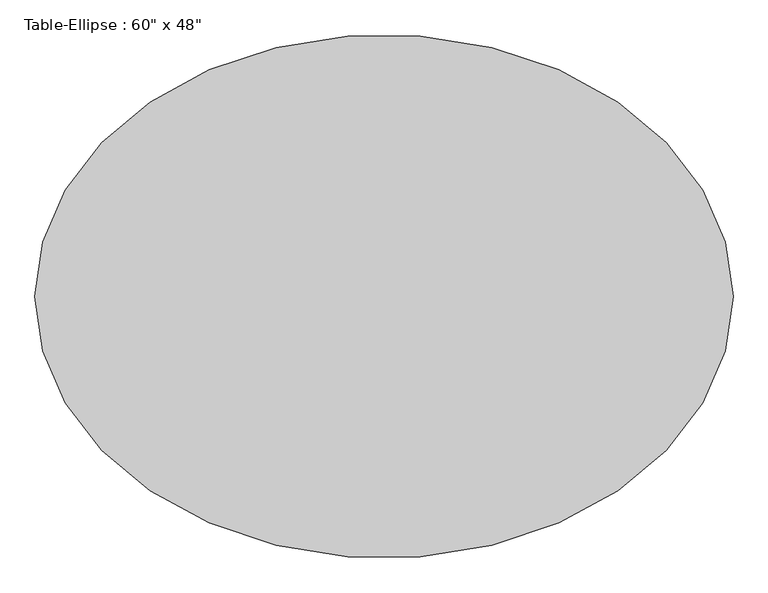
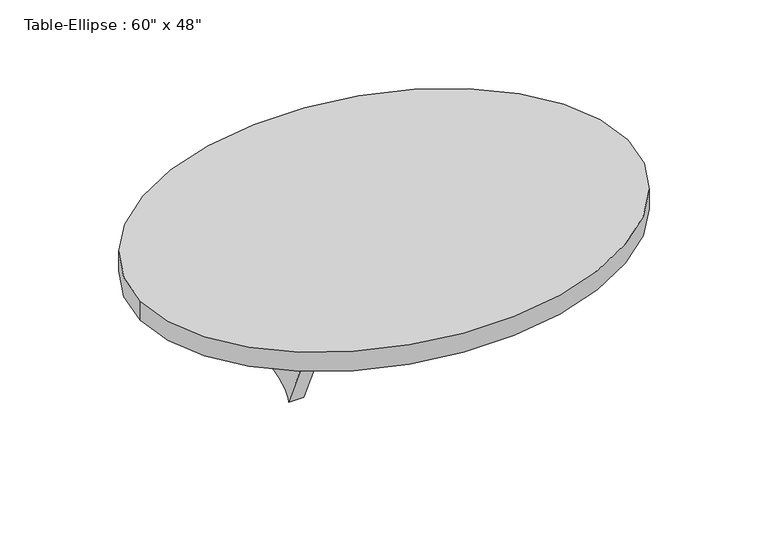
"""IFC4 building model written with IfcOpenShell, lengths in millimetres: furniture geometry."""

from ifc_helpers import new_model, si_unit, point, frame, origin, place, context, project, spatial, ellipse_curve, trimmed, source, transform, mapped, element, save
from ifc_brep_helpers import plane_surface, extruded_surface, advanced_brep


def furniture_b94c68a7(model_context):
    return source(origin(), model_context, "Body", "AdvancedBrep", [
        advanced_brep(
        [(-609.6, 0.0, 304.8), (609.6, 0.0, 304.8), (-609.6, 0.0, 254.0), (609.6, 0.0, 254.0)],
        [
            (0, 1, ellipse_curve(frame((0.0, 0.0, 304.8), z_axis=(0.0, 0.0, 1.0), x_axis=(1.0, 0.0, 0.0)), 609.6, 457.2)),
            (1, 0, ellipse_curve(frame((0.0, 0.0, 304.8), z_axis=(0.0, 0.0, 1.0), x_axis=(1.0, 0.0, 0.0)), 609.6, 457.2)),
            (2, 3, ellipse_curve(frame((0.0, 0.0, 254.0), z_axis=(0.0, 0.0, -1.0), x_axis=(1.0, 0.0, 0.0)), 609.6, 457.2)),
            (3, 2, ellipse_curve(frame((0.0, 0.0, 254.0), z_axis=(0.0, 0.0, -1.0), x_axis=(1.0, 0.0, 0.0)), 609.6, 457.2)),
            (0, 2),
            (3, 1),
        ],
        [
            plane_surface(frame((609.6, 0.0, 304.8), z_axis=(0.0, 0.0, 1.0), x_axis=(0.0, 1.0, 0.0))),
            plane_surface(frame((609.6, 0.0, 254.0), z_axis=(0.0, 0.0, -1.0), x_axis=(0.0, -1.0, 0.0))),
            extruded_surface(trimmed(ellipse_curve(frame((0.0, 0.0, 203.2), z_axis=(0.0, 0.0, 1.0), x_axis=(1.0, 0.0, 0.0)), 609.6, 457.2), [point((-609.6, 0.0, 203.2))], [point((609.6, 0.0, 203.2))], True, "CARTESIAN"), (0.0, 0.0, 50.80000000000001), 50.80000000000001),
            extruded_surface(trimmed(ellipse_curve(frame((0.0, 0.0, 203.2), z_axis=(0.0, 0.0, 1.0), x_axis=(1.0, 0.0, 0.0)), 609.6, 457.2), [point((609.6, 0.0, 203.2))], [point((-609.6, 0.0, 203.2))], True, "CARTESIAN"), (0.0, 0.0, 50.80000000000001), 50.80000000000001),
        ],
        [
            (0, [[1, 2]]),
            (1, [[3, 4]]),
            (2, [[-1, 5, -4, 6]]),
            (3, [[-2, -6, -3, -5]]),
        ],
    ),
        advanced_brep(
        [(-266.7, 228.6, 254.0), (-266.7, -228.6, 254.0), (-266.7, -114.3, 0.0), (-266.7, 114.3, 0.0), (-304.8, 228.6, 254.0), (-304.8, 114.3, 0.0), (-304.8, -114.3, 0.0), (-304.8, -228.6, 254.0)],
        [
            (0, 1),
            (1, 2),
            (2, 3, ellipse_curve(frame((-266.7, 0.0, 0.0), z_axis=(-1.0, 0.0, 0.0), x_axis=(0.0, 1.0, 0.0)), 114.3, 50.8)),
            (3, 0),
            (4, 5),
            (5, 6, ellipse_curve(frame((-304.8, 0.0, 0.0), z_axis=(1.0, 0.0, 0.0), x_axis=(0.0, 1.0, 0.0)), 114.3, 50.8)),
            (6, 7),
            (7, 4),
            (0, 4),
            (7, 1),
            (6, 2),
            (5, 3),
        ],
        [
            plane_surface(frame((-266.7, -228.6, 254.0), z_axis=(1.0, 0.0, 0.0), x_axis=(0.0, -1.0, 0.0))),
            plane_surface(frame((-304.8, -228.6, 254.0), z_axis=(-1.0, 0.0, 0.0), x_axis=(0.0, 1.0, 0.0))),
            plane_surface(frame((-266.7, 228.6, 254.0), z_axis=(0.0, 0.0, 1.0), x_axis=(-1.0, 0.0, 0.0))),
            plane_surface(frame((-266.7, -228.6, 254.0), z_axis=(0.0, -0.9119215051750983, -0.410364677328816), x_axis=(-1.0, 0.0, 0.0))),
            extruded_surface(trimmed(ellipse_curve(frame((-342.9, 0.0, 0.0), z_axis=(-1.0, 0.0, 0.0), x_axis=(0.0, 1.0, 0.0)), 114.3, 50.8), [point((-342.9, -114.3, 0.0))], [point((-342.9, 114.3, 0.0))], True, "CARTESIAN"), (38.099999999999966, 0.0, 0.0), 38.099999999999966),
            plane_surface(frame((-266.7, 114.3, 0.0), z_axis=(0.0, 0.911921505175108, -0.41036467732879445), x_axis=(-1.0, 0.0, 0.0))),
        ],
        [
            (0, [[1, 2, 3, 4]]),
            (1, [[5, 6, 7, 8]]),
            (2, [[-1, 9, -8, 10]]),
            (3, [[-2, -10, -7, 11]]),
            (4, [[-3, -11, -6, 12]]),
            (5, [[-4, -12, -5, -9]]),
        ],
    ),
        advanced_brep(
        [(304.8, 228.6, 254.0), (304.8, -228.6, 254.0), (304.8, -114.3, 0.0), (304.8, 114.3, 0.0), (266.7, 228.6, 254.0), (266.7, 114.3, 0.0), (266.7, -114.3, 0.0), (266.7, -228.6, 254.0)],
        [
            (0, 1),
            (1, 2),
            (2, 3, ellipse_curve(frame((304.8, 0.0, 0.0), z_axis=(-1.0, 0.0, 0.0), x_axis=(0.0, 1.0, 0.0)), 114.3, 50.8)),
            (3, 0),
            (4, 5),
            (5, 6, ellipse_curve(frame((266.7, 0.0, 0.0), z_axis=(1.0, 0.0, 0.0), x_axis=(0.0, 1.0, 0.0)), 114.3, 50.8)),
            (6, 7),
            (7, 4),
            (0, 4),
            (7, 1),
            (6, 2),
            (5, 3),
        ],
        [
            plane_surface(frame((304.8, -228.6, 254.0), z_axis=(1.0, 0.0, 0.0), x_axis=(0.0, -1.0, 0.0))),
            plane_surface(frame((266.7, -228.6, 254.0), z_axis=(-1.0, 0.0, 0.0), x_axis=(0.0, 1.0, 0.0))),
            plane_surface(frame((304.8, 228.6, 254.0), z_axis=(0.0, 0.0, 1.0), x_axis=(-1.0, 0.0, 0.0))),
            plane_surface(frame((304.8, -228.6, 254.0), z_axis=(0.0, -0.9119215051750985, -0.4103646773288155), x_axis=(-1.0, 0.0, 0.0))),
            extruded_surface(trimmed(ellipse_curve(frame((228.6, 0.0, 0.0), z_axis=(-1.0, 0.0, 0.0), x_axis=(0.0, 1.0, 0.0)), 114.3, 50.8), [point((228.6, -114.3, 0.0))], [point((228.6, 114.3, 0.0))], True, "CARTESIAN"), (38.099999999999994, 0.0, 0.0), 38.099999999999994),
            plane_surface(frame((304.8, 114.3, 0.0), z_axis=(0.0, 0.9119215051751104, -0.4103646773287891), x_axis=(-1.0, 0.0, 0.0))),
        ],
        [
            (0, [[1, 2, 3, 4]]),
            (1, [[5, 6, 7, 8]]),
            (2, [[-1, 9, -8, 10]]),
            (3, [[-2, -10, -7, 11]]),
            (4, [[-3, -11, -6, 12]]),
            (5, [[-4, -12, -5, -9]]),
        ],
    ),
    ])


if __name__ == "__main__":
    model = new_model("IFC4")
    model_context = context("Model", 3, world=origin())
    ifc_project = project(units=[si_unit("LENGTHUNIT", "METRE", prefix="MILLI")], contexts=[model_context])
    site = spatial("IfcSite", under=ifc_project)
    building = spatial("IfcBuilding", under=site)
    placement = place(None, origin())
    furniture_shape = furniture_b94c68a7(model_context)
    element("IfcFurniture", 1, ObjectType="Table-Ellipse : 60\" x 48\"", at=placement, inside=building, context=model_context, shape_type="MappedRepresentation", body=[
        mapped(furniture_shape, transform((0.0, 0.0, 0.0), x_axis=(1.0, 0.0, 0.0), y_axis=(0.0, 1.0, 0.0), z_axis=(0.0, 0.0, 1.0))),
    ])
    save(model, "model.ifc")

# Revit data of these elements
# Type "Table-Ellipse : 60\" x 48\""
#   Assembly Code = "E2020200"
#   Half Width = 1.5 ft
#   Half Length = 2 ft
#   Height = 1 ft
#   Length = 4 ft
#   Width = 3 ft
#   Base Material = Birch
#   Top Material = Birch
#   Default Elevation = 0
# Element 1 (IfcFurniture, "Table-Ellipse : 60\" x 48\"")
#   Materials on its faces: "Birch"
# Materials
#   "Birch": class "Wood", colour RGB 224 178 126, transparency 0, Description = "Betula Alleghaniensis", Cost = 0
